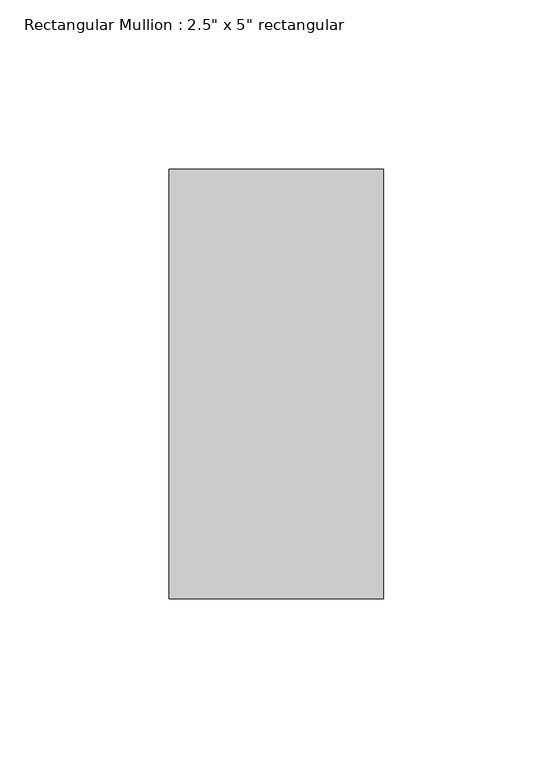
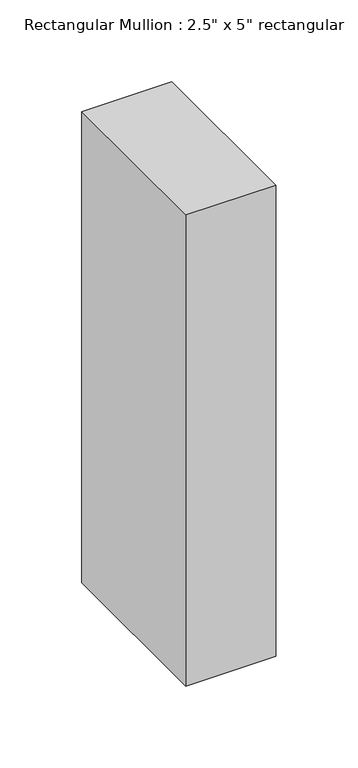
"""IFC4 building model written with IfcOpenShell, lengths in millimetres: member geometry."""

from ifc_helpers import new_model, si_unit, frame, origin, place, context, project, spatial, polyline, outline, extrude, source, transform, mapped, element, save


def member_4918008d(model_context):
    return source(origin(), model_context, "Body", "SweptSolid", [
        extrude(outline(polyline([(0.0, 63.5), (0.0, -63.5), (-63.5, -63.5), (-63.5, 63.5), (0.0, 63.5)])), frame((0.0, 0.0, -351.3666667), z_axis=(0.0, 0.0, 1.0), x_axis=(1.0, 0.0, 0.0)), (0.0, 0.0, 1.0), 351.3666667),
    ])


if __name__ == "__main__":
    model = new_model("IFC4")
    model_context = context("Model", 3, world=origin())
    ifc_project = project(units=[si_unit("LENGTHUNIT", "METRE", prefix="MILLI")], contexts=[model_context])
    site = spatial("IfcSite", under=ifc_project)
    building = spatial("IfcBuilding", under=site)
    placement = place(None, origin())
    member_shape = member_4918008d(model_context)
    element("IfcMember", 1, ObjectType="Rectangular Mullion : 2.5\" x 5\" rectangular", at=placement, inside=building, context=model_context, shape_type="MappedRepresentation", body=[
        mapped(member_shape, transform((0.0, 0.0, 0.0), x_axis=(1.0, 0.0, 0.0), y_axis=(0.0, 1.0, 0.0), z_axis=(0.0, 0.0, 1.0))),
    ])
    save(model, "model.ifc")

# Revit data of these elements
# Type "Rectangular Mullion : 2.5\" x 5\" rectangular"
#   built-in parameter 1007304 = 0.416667 (stored number, unit not read)
#   built-in parameter 1007301 = 0.104167 (stored number, unit not read)
#   built-in parameter 1007300 = 0.104167 (stored number, unit not read)
